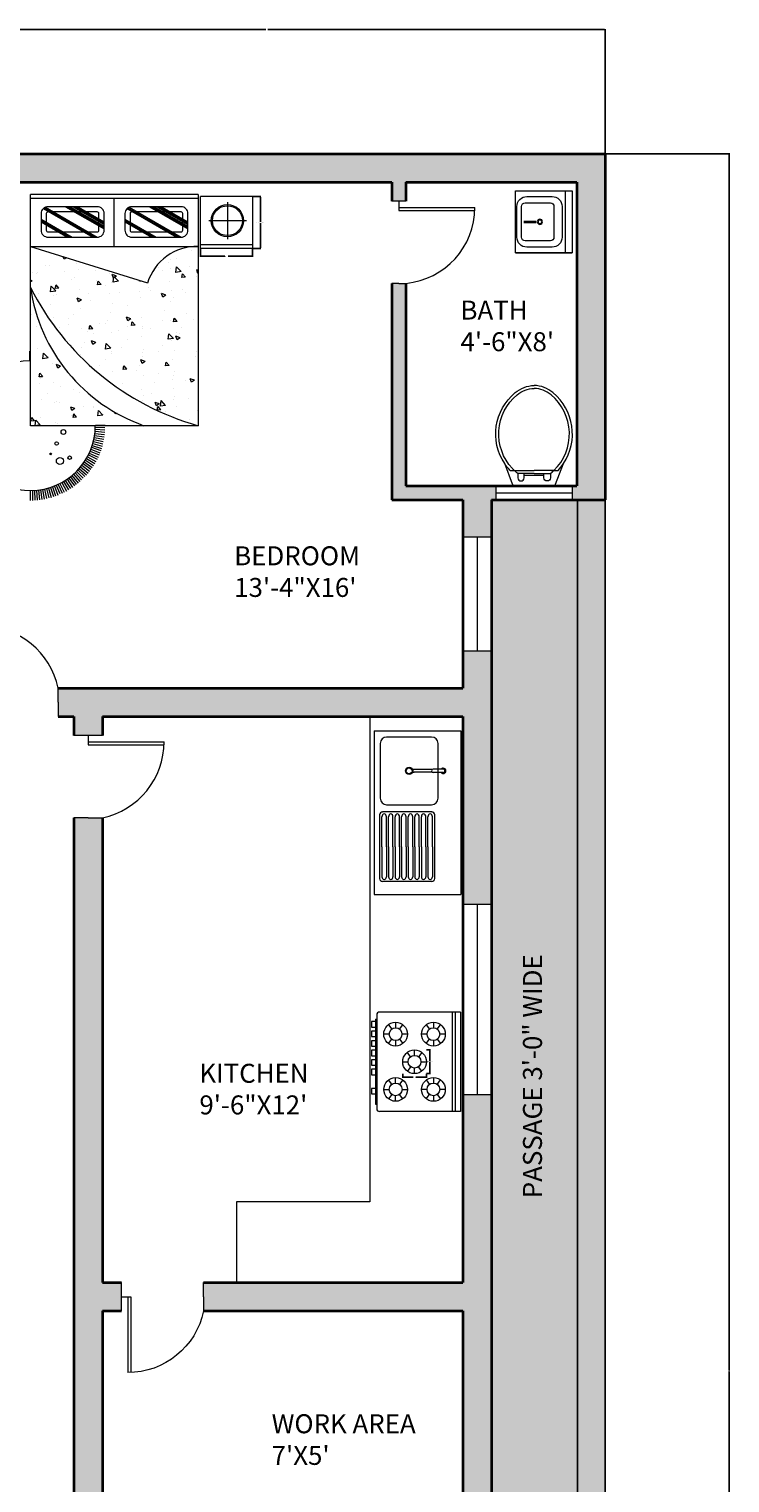
# Model space of a CAD drawing. Units: inches. Extents: x -9 to 646, y -802 to 47.
# Tile 17 of 17: x 424 to 646, y -412 to 47. Entities that reach past the tile are written whole.
import ezdxf

# ---------------------------------------------------------------- set-up
doc = ezdxf.new("R2010")
doc.units = ezdxf.units.IN
doc.header["$MEASUREMENT"] = 0
for name, color, linetype, lineweight in [('A-ANNO-DIMS', 2, 'Continuous', 18), ('A-AREA-IDEN', 7, 'Continuous', 18), ('A-DOOR', 4, 'Continuous', 18), ('A-EQPM', 8, 'Continuous', 15), ('A-FLOR-CASE', 8, 'Continuous', 18), ('A-FLOR-FIXT', 9, 'Continuous', 18), ('A-FLOR-PATT', 9, 'Continuous', 9), ('A-FURN', 8, 'Continuous', 15), ('A-FURN-PATT', 252, 'Continuous', 9), ('A-GLAZ', 4, 'Continuous', 15), ('A-WALL', 7, 'Continuous', 35), ('A-WALL-PATT', 5, 'Continuous', 9), ('C-SITE', 7, 'Continuous', 25)]:
    doc.layers.add(name, color=color, linetype=linetype, lineweight=lineweight)
doc.styles.get("Standard").update_dxf_attribs({"font": 'arial.ttf'})
doc.dimstyles.get("Standard").update_dxf_attribs({"dimtxt": 0.18, "dimasz": 0.18, "dimexe": 0.18, "dimexo": 0.0625, "dimgap": 0.09, "dimtad": 0, "dimtih": 1, "dimtoh": 1, "dimdec": 0, "dimzin": 0, "dimdsep": 46, "dimlunit": 3, "dimtxsty": 'Standard', "dimcen": 0.09, "dimadec": 0, "dimazin": 0, "dimtfac": 1, "dimtdec": 0, "dimtofl": 0, "dimtmove": 0, "dimatfit": 3, "dimfxl": 1, "dimtolj": 1, "dimtzin": 0, "dimarcsym": 0})

# ---------------------------------------------------------------- blocks, each defined once
blk = doc.blocks.new('М14 600х655')
for p, q in [((-655, 600), (-655, 0)), ((-655, 600), (-655, 0)), ((-655, 0), (-655, 600)), ((0, 600), (-655, 600)), ((0, 525), (-655, 525)), ((-165, 494), (-490, 494)), ((0, 0), (0, 600)), ((-596, 388), (-596, 121)), ((-528, 370), (-528, 103)), ((-165, 408), (-490, 408)), ((-127, 103), (-127, 370)), ((-59, 121), (-59, 388)), ((-334, 87), (-334, 220)), ((-321, 87), (-321, 220)), ((-655, 0), (-655, 0)), ((-655, 0), (-655, 0)), ((-655, 0), (0, 0)), ((-655, 0), (0, 0)), ((-490, 65), (-165, 65)), ((-490, 15), (-165, 15))]:
    blk.add_line(p, q)
for radius in [27.6, 19.3]:
    blk.add_circle((-327, 259), radius)
for centre, radius, start, end in [((-490, 388), 106, 90, 180), ((-165, 388), 106, 0, 90), ((-490, 370), 38.2, 90, 180), ((-165, 370), 38.2, 0, 90), ((-490, 121), 106, 180, 270), ((-490, 103), 38.2, 180, 270), ((-165, 121), 106, 270, 0), ((-165, 103), 38.2, 270, 0)]:
    blk.add_arc(centre, radius, start, end)
blk = doc.blocks.new('NIGHTSTAND-16_5')
for p, q in [((0, 0), (0, 16.45)), ((16.45, 16.45), (0, 16.45)), ((8.49, 14.64), (8.49, 2.96)), ((16.45, 16.45), (16.45, 0)), ((14.48, 8.8), (2.64, 8.8)), ((16.45, 1.15), (0, 1.15)), ((16.45, 0), (0, 0))]:
    blk.add_line(p, q)
for radius in [5.09, 4.73]:
    blk.add_circle((8.49, 8.8), radius)
blk = doc.blocks.new('COOKTOP-BURNER')
for p, q in [((1.48, 6.73), (2.52, 5.35)), ((3.74, 7.49), (3.74, 5.77)), ((4.97, 5.35), (6.01, 6.73)), ((1.72, 3.74), (0, 3.74)), ((1.48, 0.76), (2.52, 2.13)), ((3.74, 1.72), (3.74, 0)), ((4.97, 2.13), (6.01, 0.76)), ((7.49, 3.74), (5.76, 3.74))]:
    blk.add_line(p, q)
for radius in [3.75, 2.02]:
    blk.add_circle((3.74, 3.74), radius)
blk = doc.blocks.new('DOOR-LEAF-24-WALL9')
for p, q in [((0, 0), (0, 24)), ((1, 0), (1, 24)), ((0, 0), (1, 0))]:
    blk.add_line(p, q)
blk.add_arc((0, -0.52), 24.52, 11.8123, 90)
blk = doc.blocks.new('DOOR-LEAF-24-WALL4_5')
for p, q in [((0, 24), (24, 24)), ((0, 24), (0, 23)), ((0, 23), (24, 23))]:
    blk.add_line(p, q)
blk.add_arc((-0.11, 24), 24.12, 275.6311, 0)
blk = doc.blocks.new('GLAZING-36')
for p, q in [((0, 36), (0, 0)), ((4.5, 36), (4.5, 0)), ((9, 0), (9, 36))]:
    blk.add_line(p, q)
blk = doc.blocks.new('*D25')
at = {"layer": 'A-ANNO-DIMS', "color": 0, "lineweight": -2, "transparency": 16777216}
for p, q in [((549.88, -275.52), (551.12, -275.52)), ((550.94, -275.7), (550.94, -279.08)), ((550.94, -282.83), (550.94, -279.44)), ((549.88, -283.01), (551.12, -283.01))]:
    blk.add_line(p, q, dxfattribs=at)
at = {"layer": 'A-ANNO-DIMS', "color": 0, "transparency": 16777216}
for points in [[(550.91, -275.7), (550.97, -275.7), (550.94, -275.52)], [(550.91, -282.83), (550.97, -282.83), (550.94, -283.01)]]:
    blk.add_solid(points, dxfattribs=at)
at = {"layer": 'Defpoints', "color": 0, "transparency": 16777216}
for p in [(549.82, -275.52), (549.82, -283.01), (550.94, -283.01)]:
    blk.add_point(p, dxfattribs=at)
at = {"layer": 'A-ANNO-DIMS', "color": 0, "transparency": 16777216, "insert": (550.94, -279.26), "char_height": 0.18, "attachment_point": 5}
blk.add_mtext('\\A1;BURNER 7 TYP.', dxfattribs=at)
blk = doc.blocks.new('*D26')
at = {"layer": 'A-ANNO-DIMS', "color": 0, "lineweight": -2, "transparency": 16777216}
for p, q in [((542.33, -283.07), (542.33, -284.31)), ((542.51, -284.13), (545.62, -284.13)), ((549.64, -284.13), (546.53, -284.13)), ((549.82, -283.07), (549.82, -284.31))]:
    blk.add_line(p, q, dxfattribs=at)
at = {"layer": 'A-ANNO-DIMS', "color": 0, "transparency": 16777216}
for points in [[(542.51, -284.1), (542.51, -284.16), (542.33, -284.13)], [(549.64, -284.1), (549.64, -284.16), (549.82, -284.13)]]:
    blk.add_solid(points, dxfattribs=at)
at = {"layer": 'Defpoints', "color": 0, "transparency": 16777216}
for p in [(542.33, -283.01), (542.33, -284.13), (549.82, -283.01)]:
    blk.add_point(p, dxfattribs=at)
at = {"layer": 'A-ANNO-DIMS', "color": 0, "transparency": 16777216, "insert": (546.07, -284.13), "char_height": 0.18, "attachment_point": 5}
blk.add_mtext('\\A1;7 TYP.', dxfattribs=at)
blk = doc.blocks.new('*D45')
at = {"layer": 'A-ANNO-DIMS', "color": 0, "lineweight": -2, "transparency": 16777216}
for p, q in [((494.91, -5.59), (497.5, -5.59)), ((497.32, -5.77), (497.32, -13.63)), ((497.32, -21.86), (497.32, -14)), ((494.91, -22.04), (497.5, -22.04))]:
    blk.add_line(p, q, dxfattribs=at)
at = {"layer": 'A-ANNO-DIMS', "color": 0, "transparency": 16777216}
for points in [[(497.29, -5.77), (497.35, -5.77), (497.32, -5.59)], [(497.29, -21.86), (497.35, -21.86), (497.32, -22.04)]]:
    blk.add_solid(points, dxfattribs=at)
at = {"layer": 'Defpoints', "color": 0, "transparency": 16777216}
for p in [(494.85, -5.59), (497.32, -5.59), (494.85, -22.04)]:
    blk.add_point(p, dxfattribs=at)
at = {"layer": 'A-ANNO-DIMS', "color": 0, "transparency": 16777216, "insert": (497.32, -13.82), "char_height": 0.18, "attachment_point": 5}
blk.add_mtext('\\A1;NIGHTSTAND 16 TYP.', dxfattribs=at)
blk = doc.blocks.new('*D46')
at = {"layer": 'A-ANNO-DIMS', "color": 0, "lineweight": -2, "transparency": 16777216}
for p, q in [((478.4, -22.11), (478.4, -24.69)), ((494.85, -22.11), (494.85, -24.69)), ((478.58, -24.51), (486.11, -24.51)), ((494.67, -24.51), (487.15, -24.51))]:
    blk.add_line(p, q, dxfattribs=at)
at = {"layer": 'A-ANNO-DIMS', "color": 0, "transparency": 16777216}
for points in [[(478.58, -24.48), (478.58, -24.54), (478.4, -24.51)], [(494.67, -24.48), (494.67, -24.54), (494.85, -24.51)]]:
    blk.add_solid(points, dxfattribs=at)
at = {"layer": 'Defpoints', "color": 0, "transparency": 16777216}
for p in [(478.4, -22.04), (494.85, -22.04), (494.85, -24.51)]:
    blk.add_point(p, dxfattribs=at)
at = {"layer": 'A-ANNO-DIMS', "color": 0, "transparency": 16777216, "insert": (486.63, -24.51), "char_height": 0.18, "attachment_point": 5}
blk.add_mtext('\\A1;16 TYP.', dxfattribs=at)
blk = doc.blocks.new('*D50')
at = {"layer": 'A-ANNO-DIMS', "color": 0, "lineweight": -2, "transparency": 16777216}
for p, q in [((606.44, 7.93), (645.8, 7.93)), ((645.62, 7.75), (645.62, -376.89)), ((645.62, -761.89), (645.62, -377.25)), ((606.44, -762.07), (645.8, -762.07))]:
    blk.add_line(p, q, dxfattribs=at)
at = {"layer": 'A-ANNO-DIMS', "color": 0, "transparency": 16777216}
for points in [[(645.59, 7.75), (645.65, 7.75), (645.62, 7.93)], [(645.59, -761.89), (645.65, -761.89), (645.62, -762.07)]]:
    blk.add_solid(points, dxfattribs=at)
at = {"layer": 'Defpoints', "color": 0, "transparency": 16777216}
for p in [(606.37, 7.93), (606.37, -762.07), (645.62, -762.07)]:
    blk.add_point(p, dxfattribs=at)
at = {"layer": 'A-ANNO-DIMS', "color": 0, "transparency": 16777216, "insert": (645.62, -377.07), "char_height": 0.18, "attachment_point": 5}
blk.add_mtext('\\A1;770', dxfattribs=at)
blk = doc.blocks.new('*D53')
at = {"layer": 'A-ANNO-DIMS', "color": 0, "lineweight": -2, "transparency": 16777216}
for p, q in [((392.37, 7.99), (392.37, 47.36)), ((392.55, 47.18), (499.08, 47.18)), ((606.19, 47.18), (499.66, 47.18)), ((606.37, 7.99), (606.37, 47.36))]:
    blk.add_line(p, q, dxfattribs=at)
at = {"layer": 'A-ANNO-DIMS', "color": 0, "transparency": 16777216}
for points in [[(392.55, 47.21), (392.55, 47.15), (392.37, 47.18)], [(606.19, 47.21), (606.19, 47.15), (606.37, 47.18)]]:
    blk.add_solid(points, dxfattribs=at)
at = {"layer": 'Defpoints', "color": 0, "transparency": 16777216}
for p in [(606.37, 47.18), (392.37, 7.93), (606.37, 7.93)]:
    blk.add_point(p, dxfattribs=at)
at = {"layer": 'A-ANNO-DIMS', "color": 0, "transparency": 16777216, "insert": (499.37, 47.18), "char_height": 0.18, "attachment_point": 5}
blk.add_mtext('\\A1;214', dxfattribs=at)

msp = doc.modelspace()

# ---------------------------------------------------------------- hatches: boundary and pattern name
at = {"layer": 'A-FLOR-PATT'}
h = msp.add_hatch(dxfattribs=at)
h.set_pattern_fill('AR-HBONE', color=256)
h.paths.add_polyline_path([(597.63, -714.07), (348.37, -714.07), (348.37, -762.07), (597.63, -762.07)])
h.paths.add_polyline_path([(597.63, -101.57), (570.37, -101.57), (570.37, -496.07), (570.37, -511.17), (597.63, -511.17)])
at = {"layer": 'A-FURN-PATT'}
h = msp.add_hatch(dxfattribs=at)
h.set_pattern_fill('ANSI31', color=256, scale=2.925333, angle=105.04163, style=0)
h.paths.add_polyline_path([(429.41, -8.94), (429.38, -8.95), (429.32, -8.98), (429.25, -9.01), (429.19, -9.04), (429.12, -9.07), (429.06, -9.1), (429, -9.14), (428.94, -9.18), (428.88, -9.22), (428.82, -9.26), (428.76, -9.31), (428.71, -9.35), (428.66, -9.4), (428.6, -9.45), (428.56, -9.5), (444.11, -18.46), (445.72, -18.46), (445.87, -18.45), (445.91, -18.45)])
h = msp.add_hatch(dxfattribs=at)
h.set_pattern_fill('ANSI31', color=256, scale=2.926101, angle=105.04163, style=0)
h.paths.add_polyline_path([(437.35, -8.81), (435.54, -8.81), (447.92, -15.95), (447.92, -14.9)])
h = msp.add_hatch(dxfattribs=at)
h.set_pattern_fill('ANSI31', color=256, scale=2.9273156, angle=105.04163, style=0)
h.paths.add_polyline_path([(439.72, -8.81), (437.91, -8.81), (447.92, -14.58), (447.92, -13.53)])
h = msp.add_hatch(dxfattribs=at)
h.set_pattern_fill('ANSI31', color=256, scale=2.926313, angle=105.04163, style=0)
h.paths.add_polyline_path([(455.92, -8.94), (455.81, -8.98), (455.68, -9.04), (455.56, -9.11), (455.44, -9.19), (455.32, -9.27), (455.21, -9.36), (455.11, -9.45), (455.07, -9.5), (470.61, -18.46), (472.23, -18.46), (472.38, -18.45), (472.42, -18.45)])
h = msp.add_hatch(dxfattribs=at)
h.set_pattern_fill('ANSI31', color=256, scale=2.927018, angle=105.04163, style=0)
h.paths.add_polyline_path([(463.86, -8.81), (462.04, -8.81), (474.42, -15.95), (474.42, -14.9)])
h = msp.add_hatch(dxfattribs=at)
h.set_pattern_fill('ANSI31', color=256, scale=2.9233957, angle=105.04163, style=0)
h.paths.add_polyline_path([(466.23, -8.81), (464.42, -8.81), (474.42, -14.58), (474.42, -13.53)])
h = msp.add_hatch(dxfattribs=at)
h.set_pattern_fill('ANSI31', color=256, scale=2.9260728, angle=105.04163, style=0)
h.paths.add_polyline_path([(427.96, -12.69), (427.96, -13.74), (436.15, -18.46), (437.97, -18.46)])
h = msp.add_hatch(dxfattribs=at)
h.set_pattern_fill('ANSI31', color=256, scale=2.9270259, angle=105.04163, style=0)
h.paths.add_polyline_path([(454.47, -12.69), (454.47, -13.74), (462.66, -18.46), (464.48, -18.46)])
h = msp.add_hatch(dxfattribs=at)
h.set_pattern_fill('AR-CONC', color=256, scale=0.073127, angle=180, style=0)
h.set_pattern_definition([(130, (1102.287, -4154.876), (-13.322528, -1.16557), [1.39306, -15.32366]), (185, (1102.287, -4154.876), (2.577185, 13.971305), [1.11445, -12.258928]), (79.549, (1101.176, -4154.974), (-10.74539, 12.80567), [1.18392, -13.0231]), (133.8158, (1102.287, -4151.162), (-19.823063, -3.07441), [2.08959, -22.98549]), (83.3644, (1100.635, -4151.418), (-17.36054, 18.09337), [1.77588, -19.53465]), (188.816, (1102.287, -4151.162), (-17.36057, 18.09333), [1.67167, -18.38839]), (159, (1100.429, -4152.09), (-11.087067, -7.47832), [1.39306, -15.32366]), (214, (1100.429, -4152.09), (-4.519366, 13.469023), [1.11445, -12.258928]), (108.5486, (1099.505, -4152.713), (-15.606403, 5.990732), [1.18392, -13.0231]), (142.5, (1102.2865, -4154.8764), (-0.225859, 6.1832147), [0, -12.110335, 0, -12.444669, 0, -12.305363]), (172.5, (1102.2865, -4154.8764), (-4.886289, 7.325856), [0, -7.095319, 0, -11.831723, 0, -4.689969]), (212.5, (1106.4286, -4154.8764), (-9.9152666, -0.418923), [0, -4.643533, 0, -14.487824, 0, -19.224227]), (222.5, (1108.286, -4154.876), (-10.83217, 1.85935), [0, -6.036593, 0, -9.6214, 0, -13.651988])])
edge = h.paths.add_edge_path()
edge.add_ellipse((477.28, -37.72), major_axis=(-11.56, 11.56), ratio=1, start_angle=-43.8468, end_angle=28.0453, ccw=False)
edge.add_line((476.95, -21.38), (477.61, -21.38))
edge.add_line((477.61, -21.38), (477.61, -78.08))
edge.add_ellipse((500.9, 4.17), major_axis=(-60.45, 60.45), ratio=1, start_angle=71.7955, end_angle=119.1914, ccw=False)
edge.add_line((424.59, -34.37), (424.59, -21.38))
edge.add_line((424.59, -21.38), (461.64, -32.95))
edge = h.paths.add_edge_path()
edge.add_line((460.51, -78.08), (424.59, -78.08))
edge.add_line((424.59, -78.08), (424.59, -34.37))
edge.add_ellipse((478.71, -26.51), major_axis=(38.67, 38.67), ratio=1, start_angle=143.2583, end_angle=205.5572)
at = {"layer": 'A-WALL-PATT'}
h = msp.add_hatch(color=256, dxfattribs=at)
h.dxf.hatch_style = 1
h.paths.add_polyline_path([(73.4, -418.07), (63.37, -418.07), (63.37, -487.07), (63.35, -496.07), (67.87, -496.07), (67.87, -427.07), (73.4, -427.07)])
h.paths.add_polyline_path([(73.87, -487.07), (67.87, -487.07), (67.87, -496.07), (73.87, -496.07)])
h.paths.add_polyline_path([(39.37, -496.07), (39.35, -496.07), (39.35, -487.07), (30.37, -487.07), (30.37, -646.07), (69.62, -646.07), (69.62, -637.07), (39.37, -637.07)])
h.paths.add_polyline_path([(158.27, -637.07), (105.62, -637.07), (105.62, -646.07), (158.27, -646.07)])
h.paths.add_polyline_path([(286.47, -637.07), (194.27, -637.07), (194.27, -646.07), (286.47, -646.07)])
h.paths.add_polyline_path([(357.37, -552.07), (352.87, -552.07), (348.37, -552.07), (348.37, -637.07), (322.47, -637.07), (322.47, -646.07), (357.37, -646.07)])
h.paths.add_polyline_path([(357.37, -459.07), (352.87, -459.07), (348.37, -459.07), (348.37, -526.07), (357.37, -526.07), (357.37, -520.07), (363.37, -520.07), (363.37, -511.07), (357.37, -511.07)], flags=17)
h.paths.add_polyline_path([(39.37, -262.07), (213.37, -262.07), (213.37, -268.07), (222.37, -268.07), (222.37, -247.07), (213.37, -247.07), (213.37, -253.07), (39.37, -253.07), (39.37, -1.07), (222.37, -1.07), (222.37, 7.93), (30.37, 7.93), (30.37, -427.07), (39.36, -427.07), (39.36, -418.07)])
h.paths.add_polyline_path([(570.37, -149.32), (561.37, -149.32), (561.37, -161.07), (433.37, -161.07), (433.37, -165.57), (433.37, -170.07), (438.37, -170.07), (438.37, -176.07), (447.37, -176.07), (447.37, -170.07), (561.37, -170.07), (561.37, -229.57), (570.37, -229.57)])
h.paths.add_polyline_path([(570.37, -289.57), (561.37, -289.57), (561.37, -349.07), (479.37, -349.07), (479.37, -353.57), (479.37, -358.07), (561.37, -358.07), (561.37, -418.07), (447.37, -418.07), (447.37, -358.07), (453.37, -358.07), (453.37, -349.07), (447.37, -349.07), (447.37, -202.07), (442.87, -202.07), (438.37, -202.07), (438.37, -427.07), (561.37, -427.07), (561.37, -451.07), (570.37, -451.07)])
h.paths.add_polyline_path([(570.37, -496.07), (570.37, -487.07), (561.37, -487.07), (561.37, -511.07), (411.37, -511.07), (411.37, -515.57), (411.37, -520.07), (570.37, -520.07)])
h = msp.add_hatch(color=256, dxfattribs=at)
h.dxf.hatch_style = 1
h.paths.add_polyline_path([(401.37, -1.07), (538.87, -1.07), (538.87, -7.07), (543.37, -7.07), (543.37, -1.07), (597.37, -1.07), (597.37, -97.07), (595.89, -97.07), (595.89, -101.57), (606.37, -101.57), (606.37, 7.93), (570.37, 7.93), (392.37, 7.93), (392.37, -1.07), (392.37, -31.07), (337.37, -31.07), (337.37, -35.57), (392.37, -35.57), (392.37, -161.07), (254.37, -161.07), (254.37, -165.57), (254.37, -170.07), (401.37, -170.07)])
h.paths.add_polyline_path([(228.37, -161.07), (222.37, -161.07), (222.37, -35.57), (277.37, -35.57), (277.37, -31.07), (222.37, -31.07), (222.37, -28.07), (213.37, -28.07), (213.37, -221.07), (217.87, -221.07), (222.37, -221.07), (222.37, -170.07), (228.37, -170.07)])
h.paths.add_polyline_path([(571.89, -97.07), (543.37, -97.07), (543.37, -33.07), (541.12, -33.07), (538.87, -33.07), (538.87, -101.57), (561.37, -101.57), (561.37, -113.32), (570.37, -113.32), (570.37, -101.57), (571.89, -101.57)], flags=17)
h = msp.add_hatch(color=256, dxfattribs=at)
h.dxf.hatch_style = 1
h.paths.add_polyline_path([(597.63, -101.57), (570.37, -101.57), (570.37, -496.07), (570.37, -511.17), (597.63, -511.17)], flags=0)
h.paths.add_polyline_path([(606.37, -101.57), (597.63, -101.57), (597.63, -511.17), (570.37, -511.17), (570.37, -513.2), (597.63, -513.2), (597.63, -712.07), (606.37, -712.07)])

# ---------------------------------------------------------------- linework, layer by layer
at = {"layer": 'A-DOOR'}
for p, q in [((543.37, -7.07), (538.87, -7.07)), ((541.12, -7.07), (541.12, -9.07)), ((541.12, -33.07), (538.87, -33.07)), ((541.12, -33.07), (543.37, -33.07)), ((433.37, -165.57), (433.37, -161.07)), ((433.37, -165.57), (433.37, -170.07)), ((447.37, -176.07), (438.37, -176.07)), ((442.87, -176.07), (442.87, -178.07)), ((442.87, -202.07), (438.37, -202.07)), ((442.87, -202.07), (447.37, -202.07)), ((453.37, -358.07), (453.37, -349.07)), ((479.37, -353.57), (479.37, -349.07)), ((453.37, -353.57), (455.37, -353.57)), ((479.37, -353.57), (479.37, -358.07))]:
    msp.add_line(p, q, dxfattribs=at)
at = {"layer": 'A-EQPM'}
for p, q in [((533.68, -266.56), (532.49, -266.56)), ((532.49, -266.56), (532.49, -268.3)), ((533.68, -265.81), (533.68, -292.72)), ((533.68, -265.81), (534.11, -265.81)), ((534.11, -264.39), (534.11, -294.14)), ((560.62, -263.53), (534.98, -263.53)), ((558.03, -263.53), (558.03, -295)), ((558.89, -263.53), (558.89, -295)), ((560.62, -263.53), (560.62, -295)), ((532.49, -268.3), (533.68, -268.3)), ((532.49, -269.57), (532.49, -271.32)), ((533.68, -269.57), (532.49, -269.57)), ((532.49, -271.32), (533.68, -271.32)), ((532.49, -272.59), (532.49, -274.34)), ((533.68, -272.59), (532.49, -272.59)), ((532.49, -274.34), (533.68, -274.34)), ((532.49, -275.61), (532.49, -277.35)), ((533.68, -275.61), (532.49, -275.61)), ((532.49, -277.35), (533.68, -277.35)), ((532.49, -278.62), (532.49, -280.37)), ((533.68, -278.62), (532.49, -278.62)), ((532.49, -280.37), (533.68, -280.37)), ((532.49, -281.64), (532.49, -283.38)), ((533.68, -281.64), (532.49, -281.64)), ((532.49, -283.38), (533.68, -283.38)), ((532.49, -287.67), (532.49, -289.42)), ((533.68, -287.67), (532.49, -287.67)), ((532.49, -289.42), (533.68, -289.42)), ((533.68, -292.72), (534.11, -292.72)), ((560.62, -295), (534.98, -295))]:
    msp.add_line(p, q, dxfattribs=at)
for centre, start, end in [((534.98, -264.39), 90, 180), ((534.98, -294.14), 180, 270)]:
    msp.add_arc(centre, 0.862, start, end, dxfattribs=at)
at = {"layer": 'A-FLOR-CASE'}
for p, q in [((531.97, -170.07), (531.97, -323.56)), ((531.97, -323.56), (489.8, -323.56)), ((489.8, -323.56), (489.8, -349.07))]:
    msp.add_line(p, q, dxfattribs=at)
at = {"layer": 'A-FLOR-FIXT'}
for p, q in [((576.31, -92.27), (577.65, -92.27)), ((577.65, -92.27), (583.89, -92.27)), ((590.13, -92.27), (583.89, -92.27)), ((590.13, -92.27), (591.46, -92.27)), ((533.32, -174.57), (560.69, -174.57)), ((533.32, -174.57), (533.32, -226.36)), ((560.69, -174.57), (560.69, -226.36)), ((535.22, -178.59), (535.22, -195.91)), ((551.49, -176.55), (537.26, -176.55)), ((553.53, -187.57), (553.53, -178.59)), ((553.53, -195.91), (553.53, -187.82)), ((535.02, -201.21), (535.02, -221.31)), ((535.77, -211.26), (535.77, -201.77)), ((551.54, -200.26), (535.96, -200.26)), ((537.18, -211.26), (537.18, -201.77)), ((537.26, -197.95), (551.49, -197.95)), ((537.84, -211.26), (537.84, -201.77)), ((539.26, -211.26), (539.26, -201.77)), ((539.92, -211.26), (539.92, -201.77)), ((541.34, -211.26), (541.34, -201.77)), ((542, -211.26), (542, -201.77)), ((543.42, -211.26), (543.42, -201.77)), ((544.08, -211.26), (544.08, -201.77)), ((545.5, -211.26), (545.5, -201.77)), ((546.16, -211.26), (546.16, -201.77)), ((547.57, -211.26), (547.57, -201.77)), ((548.24, -211.26), (548.24, -201.77)), ((549.65, -211.26), (549.65, -201.77)), ((550.32, -211.26), (550.32, -201.77)), ((551.73, -211.26), (551.73, -201.77)), ((552.49, -221.31), (552.49, -201.21)), ((535.77, -211.26), (535.77, -220.74)), ((537.18, -211.26), (537.18, -220.74)), ((537.84, -211.26), (537.84, -220.74)), ((539.26, -211.26), (539.26, -220.74)), ((539.92, -211.26), (539.92, -220.74)), ((541.34, -211.26), (541.34, -220.74)), ((542, -211.26), (542, -220.74)), ((543.42, -211.26), (543.42, -220.74)), ((544.08, -211.26), (544.08, -220.74)), ((545.5, -211.26), (545.5, -220.74)), ((546.16, -211.26), (546.16, -220.74)), ((547.57, -211.26), (547.57, -220.74)), ((548.24, -211.26), (548.24, -220.74)), ((549.65, -211.26), (549.65, -220.74)), ((550.32, -211.26), (550.32, -220.74)), ((551.73, -211.26), (551.73, -220.74)), ((551.54, -222.25), (535.96, -222.25)), ((533.32, -226.36), (560.69, -226.36))]:
    msp.add_line(p, q, dxfattribs=at)
for points in [[(574.6, -90.09, -0.383919), (577.92, -67.62, -0.163732), (583.89, -65.34, -0.359733)], [(577.01, -91.62, -0.431639), (578.53, -68.35, -0.162618), (583.89, -66.29, -0.470877)], [(593.18, -90.09, 0.383919), (589.85, -67.62, 0.163732), (583.89, -65.34, 0.359733)], [(590.13, -92.27, 0.448546), (589.25, -68.35, 0.162618), (583.89, -66.29, 0.470877)], [(576.31, -92.27, -0.040937), (574.6, -90.09, -0.163732)], [(583.89, -97.07), (577.83, -97.07, -0.31031), (577.09, -96.56), (574.6, -90.09, -0.209071)], [(577.65, -92.27, -0.014165), (577.01, -91.62, -0.162618)], [(583.89, -97.07), (589.95, -97.07, 0.31031), (590.69, -96.56), (593.18, -90.09, 0.209071)], [(591.46, -92.27, 0.040937), (593.18, -90.09, 0.163732)], [(578.74, -93.22, -0.022712), (577.65, -92.27, -0.162618)], [(583.89, -93.22), (578.74, -93.22, -0.022712)], [(578.74, -93.22), (578.74, -94.56, 1), (580.76, -94.56), (580.76, -93.86)], [(583.89, -93.22), (589.04, -93.22, 0.476108)], [(589.04, -93.22), (589.04, -94.56, -1), (587.01, -94.56), (587.01, -93.86)], [(589.04, -93.22, 0.022712), (590.13, -92.27, 0.162618)]]:
    msp.add_lwpolyline(points, format="xyb", dxfattribs=at)
for points in [[(580.76, -93.86), (580.76, -93.22)], [(587.01, -93.86), (580.76, -93.86)], [(587.01, -93.86), (587.01, -93.22)], [(551.65, -186.83), (545.92, -186.83)], [(551.65, -187.67), (545.92, -187.67)], [(555.12, -186.68), (552.01, -186.68)], [(555.12, -187.82), (552.01, -187.82)]]:
    msp.add_lwpolyline(points, dxfattribs=at)
for radius in [1.18, 0.944]:
    msp.add_circle((544.37, -187.25), radius, dxfattribs=at)
for centre, radius, start, end in [((537.26, -178.59), 2.04, 90, 180), ((551.49, -178.59), 2.04, 0, 90), ((545.88, -187.25), 0.426, 84.9463, 275.0537), ((552.03, -187.25), 0.567, 92.2198, 267.7802), ((555.12, -187.25), 0.848, 221.9018, 138.0982), ((555.12, -187.25), 0.566, 270, 90), ((537.26, -195.91), 2.04, 180, 270), ((551.49, -195.91), 2.04, 270, 0), ((535.96, -201.21), 0.944, 90, 180), ((536.71, -201.77), 0.944, 104.4903, 180), ((536.24, -201.77), 0.944, 0, 75.5097), ((538.79, -201.77), 0.944, 104.4903, 180), ((538.32, -201.77), 0.944, 0, 75.5097), ((540.87, -201.77), 0.944, 104.4903, 180), ((540.39, -201.77), 0.944, 0, 75.5097), ((542.95, -201.77), 0.944, 104.4903, 180), ((542.47, -201.77), 0.944, 0, 75.5097), ((545.02, -201.77), 0.944, 104.4903, 180), ((544.55, -201.77), 0.944, 0, 75.5097), ((547.1, -201.77), 0.944, 104.4903, 180), ((546.63, -201.77), 0.944, 0, 75.5097), ((549.18, -201.77), 0.944, 104.4903, 180), ((548.71, -201.77), 0.944, 0, 75.5097), ((551.26, -201.77), 0.944, 104.4903, 180), ((550.79, -201.77), 0.944, 0, 75.5097), ((551.54, -201.21), 0.944, 0, 90), ((535.96, -221.31), 0.944, 180, 270), ((536.71, -220.74), 0.944, 180, 255.5097), ((536.24, -220.74), 0.944, 284.4903, 0), ((538.79, -220.74), 0.944, 180, 255.5097), ((538.32, -220.74), 0.944, 284.4903, 0), ((540.87, -220.74), 0.944, 180, 255.5097), ((540.39, -220.74), 0.944, 284.4903, 0), ((542.95, -220.74), 0.944, 180, 255.5097), ((542.47, -220.74), 0.944, 284.4903, 0), ((545.02, -220.74), 0.944, 180, 255.5097), ((544.55, -220.74), 0.944, 284.4903, 0), ((547.1, -220.74), 0.944, 180, 255.5097), ((546.63, -220.74), 0.944, 284.4903, 0), ((549.18, -220.74), 0.944, 180, 255.5097), ((548.71, -220.74), 0.944, 284.4903, 0), ((551.26, -220.74), 0.944, 180, 255.5097), ((550.79, -220.74), 0.944, 284.4903, 0), ((551.54, -221.31), 0.944, 270, 0)]:
    msp.add_arc(centre, radius, start, end, dxfattribs=at)
at = {"layer": 'A-FURN'}
for p, q in [((424.59, -78.08), (424.59, -4.96)), ((477.61, -4.96), (424.59, -4.96)), ((424.59, -6.15), (477.61, -6.15)), ((451.1, -21.38), (451.1, -6.15)), ((477.61, -4.96), (477.61, -78.08)), ((424.59, -21.38), (477.61, -21.38)), ((424.59, -21.38), (461.64, -32.95)), ((424.42, -57.55), (424.42, -54.5)), ((477.61, -78.08), (424.59, -78.08)), ((445.12, -77.91), (448.18, -77.91)), ((444.66, -82.42), (447.64, -83.09)), ((444.79, -81.78), (447.79, -82.36)), ((444.89, -81.14), (447.91, -81.62)), ((444.98, -80.5), (448.01, -80.88)), ((445.05, -79.85), (448.09, -80.14)), ((445.09, -79.2), (448.14, -79.4)), ((445.12, -78.55), (448.17, -78.65)), ((442.94, -87.3), (445.65, -88.7)), ((443.22, -86.72), (445.98, -88.03)), ((443.48, -86.12), (446.28, -87.35)), ((443.73, -85.52), (446.56, -86.65)), ((443.95, -84.91), (446.82, -85.96)), ((444.16, -84.3), (447.06, -85.25)), ((444.35, -83.68), (447.28, -84.53)), ((444.51, -83.05), (447.47, -83.81)), ((440.04, -91.6), (442.33, -93.63)), ((440.46, -91.11), (442.81, -93.06)), ((440.87, -90.6), (443.27, -92.48)), ((441.26, -90.08), (443.72, -91.88)), ((441.63, -89.54), (444.15, -91.27)), ((441.98, -89), (444.55, -90.65)), ((442.32, -88.44), (444.94, -90.01)), ((442.64, -87.88), (445.31, -89.36)), ((433.94, -96.36), (435.3, -99.09)), ((434.51, -96.06), (435.96, -98.75)), ((435.07, -95.74), (436.61, -98.38)), ((435.63, -95.4), (437.25, -97.99)), ((436.17, -95.04), (437.87, -97.58)), ((436.7, -94.66), (438.48, -97.15)), ((437.22, -94.27), (439.07, -96.7)), ((437.72, -93.87), (439.66, -96.23)), ((438.22, -93.44), (440.22, -95.74)), ((438.69, -93), (440.77, -95.24)), ((439.16, -92.55), (441.31, -94.72)), ((439.61, -92.08), (441.82, -94.18)), ((424.56, -98.61), (424.52, -101.72)), ((425.2, -98.6), (425.27, -101.7)), ((425.85, -98.57), (426.02, -101.67)), ((426.5, -98.52), (426.76, -101.61)), ((427.15, -98.45), (427.5, -101.52)), ((427.79, -98.36), (428.24, -101.41)), ((428.43, -98.25), (428.98, -101.28)), ((429.06, -98.12), (429.71, -101.13)), ((429.7, -97.97), (430.43, -100.95)), ((430.32, -97.8), (431.15, -100.75)), ((430.94, -97.61), (431.87, -100.53)), ((431.56, -97.4), (432.57, -100.29)), ((432.16, -97.17), (433.27, -100.02)), ((432.76, -96.92), (433.85, -99.48)), ((433.35, -96.65), (434.63, -99.42))]:
    msp.add_line(p, q, dxfattribs=at)
for points in [[(445.72, -8.81), (430.16, -8.81, 0.414214), (427.96, -11), (427.96, -16.26, 0.414214), (430.16, -18.46), (445.72, -18.46, 0.414214), (447.92, -16.26), (447.92, -11, 0.414214)], [(472.23, -8.81), (456.66, -8.81, 0.414214), (454.47, -11), (454.47, -16.26, 0.414214), (456.66, -18.46), (472.23, -18.46, 0.414214), (474.42, -16.26), (474.42, -11, 0.414214)], [(445.72, -10.46), (430.16, -10.46, 0.414214), (429.61, -11), (429.61, -16.26, 0.414214), (430.16, -16.81), (445.72, -16.81, 0.414214), (446.27, -16.26), (446.27, -11, 0.414214)], [(472.23, -10.46), (456.66, -10.46, 0.414214), (456.12, -11), (456.12, -16.26, 0.414214), (456.66, -16.81), (472.23, -16.81, 0.414214), (472.78, -16.26), (472.78, -11, 0.414214)]]:
    msp.add_lwpolyline(points, format="xyb", close=True, dxfattribs=at)
for centre, radius in [((435.03, -80.08), 0.754), ((431.01, -86.99), 0.269), ((432.88, -83.73), 0.557), ((433.9, -89.24), 1.11), ((436.99, -88.22), 0.557)]:
    msp.add_circle(centre, radius, dxfattribs=at)
for centre, radius, start, end in [((477.28, -37.72), 16.35, 88.8468, 163.0453), ((500.9, 4.17), 85.48, 206.7955, 254.1914), ((478.71, -26.51), 54.69, 188.2583, 250.5572), ((424.59, -78.08), 20.53, 90.4973, 0.4973)]:
    msp.add_arc(centre, radius, start, end, dxfattribs=at)
at = {"layer": 'A-GLAZ'}
for p, q in [((571.89, -97.07), (595.89, -97.07)), ((571.89, -101.57), (571.89, -97.07)), ((571.89, -99.32), (595.89, -99.32)), ((595.89, -97.07), (595.89, -101.57)), ((595.89, -101.57), (571.89, -101.57)), ((561.37, -113.32), (561.37, -113.32)), ((570.37, -113.32), (561.37, -113.32)), ((561.37, -149.32), (570.37, -149.32)), ((561.37, -229.57), (561.37, -289.57)), ((570.37, -229.57), (561.37, -229.57)), ((565.87, -229.57), (565.87, -289.57)), ((570.37, -289.57), (570.37, -229.57)), ((561.37, -289.57), (570.37, -289.57))]:
    msp.add_line(p, q, dxfattribs=at)
at = {"layer": 'A-WALL'}
for p, q in [((30.37, 7.93), (570.37, 7.93)), ((570.37, 7.93), (606.37, 7.93)), ((606.37, 7.93), (606.37, -101.57)), ((401.37, -1.07), (538.87, -1.07)), ((538.87, -1.07), (538.87, -7.07)), ((543.37, -1.07), (543.37, -7.07)), ((543.37, -1.07), (597.37, -1.07)), ((597.37, -1.07), (597.37, -97.07)), ((538.87, -33.07), (538.87, -101.57)), ((543.37, -33.07), (543.37, -97.07)), ((543.37, -97.07), (597.37, -97.07)), ((538.87, -101.57), (561.37, -101.57)), ((561.37, -101.57), (561.37, -161.07)), ((570.37, -101.57), (570.37, -496.07)), ((570.37, -101.57), (606.37, -101.57)), ((433.37, -161.07), (561.37, -161.07)), ((433.37, -170.07), (438.37, -170.07)), ((438.37, -170.07), (438.37, -176.07)), ((447.37, -170.07), (447.37, -176.07)), ((447.37, -170.07), (561.37, -170.07)), ((561.37, -170.07), (561.37, -349.07)), ((438.37, -202.07), (438.37, -427.07)), ((447.37, -202.07), (447.37, -349.07)), ((447.37, -349.07), (453.37, -349.07)), ((479.37, -349.07), (561.37, -349.07)), ((447.37, -358.07), (453.37, -358.07)), ((447.37, -358.07), (447.37, -418.07)), ((479.37, -358.07), (561.37, -358.07)), ((561.37, -358.07), (561.37, -418.07))]:
    msp.add_line(p, q, dxfattribs=at)
at = {"layer": 'C-SITE'}
for p, q in [((597.63, -101.57), (597.63, -511.17)), ((606.37, -101.57), (606.37, -762.07))]:
    msp.add_line(p, q, dxfattribs=at)

# ---------------------------------------------------------------- block references
at = {"layer": 'A-DOOR'}
for name, p in [('DOOR-LEAF-24-WALL4_5', (541.12, -33.07)), ('DOOR-LEAF-24-WALL9', (409.37, -165.57))]:
    msp.add_blockref(name, p, dxfattribs=at)
at = {"layer": 'A-DOOR', "rotation": 270.0000000000001}
msp.add_blockref('DOOR-LEAF-24-WALL9', (442.87, -178.07), dxfattribs=at)
at = {"layer": 'A-DOOR', "extrusion": (0, 0, -1), "zscale": -1, "rotation": 180}
msp.add_blockref('DOOR-LEAF-24-WALL9', (-455.37, -353.57), dxfattribs=at)
at = {"layer": 'A-EQPM'}
for p in [(536.35, -274.27), (548.31, -274.27), (548.31, -291.75)]:
    msp.add_blockref('COOKTOP-BURNER', p, dxfattribs=at)
at = {"layer": 'A-EQPM', "rotation": 180}
for p in [(549.82, -275.52), (543.84, -284.26)]:
    msp.add_blockref('COOKTOP-BURNER', p, dxfattribs=at)
at = {"layer": 'A-FLOR-FIXT', "xscale": -0.0298457359050645, "yscale": 0.0298457359050645, "zscale": 0.0298457359050645, "rotation": 270}
msp.add_blockref('М14 600х655', (578, -3.84), dxfattribs=at)
at = {"layer": 'A-FURN'}
msp.add_blockref('NIGHTSTAND-16_5', (478.4, -22.04), dxfattribs=at)
at = {"layer": 'A-GLAZ'}
msp.add_blockref('GLAZING-36', (561.37, -149.32), dxfattribs=at)

# ---------------------------------------------------------------- texts
at = {"layer": 'A-AREA-IDEN', "char_height": 6, "attachment_point": 1}
for s, insert in [('BATH\\P4\'-6"X8\'', (560.61, -38.52)), ('BEDROOM\\P13\'-4"X16\'', (489.04, -116.24)), ('KITCHEN\\P9\'-6"X12\'', (478.03, -279.91)), ("WORK AREA\\P7'X5'", (500.89, -390.76))]:
    msp.add_mtext(s, dxfattribs=dict(at, insert=insert))
at = {"layer": 'A-AREA-IDEN', "insert": (580.38, -322.41), "char_height": 6, "attachment_point": 1, "rotation": 90}
msp.add_mtext('PASSAGE 3\'-0" WIDE', dxfattribs=at)

# ---------------------------------------------------------------- dimensions: what is measured, and where the dimension line sits
at = {"layer": 'A-ANNO-DIMS'}
dim = msp.add_linear_dim(base=(606.37, 47.18), p1=(392.37, 7.93), p2=(606.37, 7.93), dimstyle='Standard', override={"dimdec": 0, "dimlfac": 1, "dimrnd": 0, "dimzin": 0, "dimdsep": 46, "dimlunit": 2}, dxfattribs=at)
dim.commit()
dim.dimension.update_dxf_attribs({"geometry": '*D53', "text_midpoint": (499.37, 47.18)})
dim = msp.add_linear_dim(base=(645.62, -762.07), p1=(606.37, 7.93), p2=(606.37, -762.07), angle=90, dimstyle='Standard', override={"dimdec": 0, "dimlfac": 1, "dimrnd": 0, "dimzin": 0, "dimdsep": 46, "dimlunit": 2}, dxfattribs=at)
dim.commit()
dim.dimension.update_dxf_attribs({"geometry": '*D50', "text_midpoint": (645.62, -377.07)})
for base, p1, p2, angle, text, picture, middle in [((497.32, -5.59), (494.85, -22.04), (494.85, -5.59), 90, 'NIGHTSTAND <> TYP.', '*D45', (497.32, -13.82)), ((550.94, -283.01), (549.82, -275.52), (549.82, -283.01), 270, 'BURNER <> TYP.', '*D25', (550.94, -279.26)), ((542.33, -284.13), (549.82, -283.01), (542.33, -283.01), 180, '<> TYP.', '*D26', (546.07, -284.13))]:
    dim = msp.add_linear_dim(base=base, p1=p1, p2=p2, angle=angle, text=text, dimstyle='Standard', override={"dimdec": 0, "dimlfac": 1, "dimrnd": 0, "dimzin": 0, "dimdsep": 46, "dimlunit": 2}, dxfattribs=at)
    dim.commit()
    dim.dimension.update_dxf_attribs({"geometry": picture, "text_midpoint": middle})
dim = msp.add_linear_dim(base=(494.85, -24.51), p1=(478.4, -22.04), p2=(494.85, -22.04), text='<> TYP.', dimstyle='Standard', override={"dimdec": 0, "dimlfac": 1, "dimrnd": 0, "dimzin": 0, "dimdsep": 46, "dimlunit": 2}, dxfattribs=at)
dim.commit()
dim.dimension.update_dxf_attribs({"geometry": '*D46', "text_midpoint": (486.63, -24.51)})

doc.saveas('drawing.dxf')
